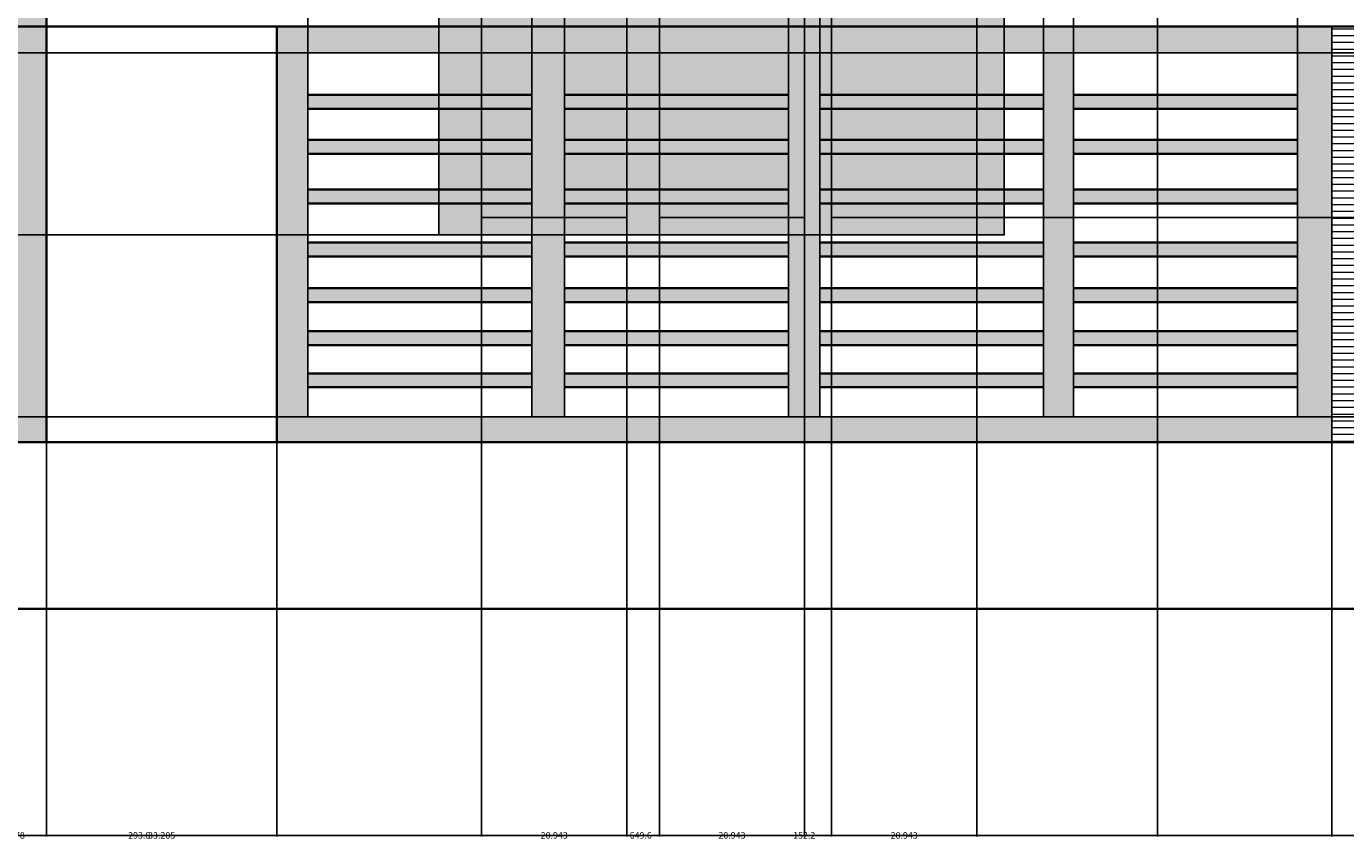
# Model space of a CAD drawing. Units: inches. Extents: x -5 to 714, y 84 to 644.
# Tile 5 of 20: x 266 to 457, y 84 to 201. Entities that reach past the tile are written whole.
import ezdxf

# ---------------------------------------------------------------- set-up
doc = ezdxf.new("R2010")
doc.units = ezdxf.units.IN
doc.header["$MEASUREMENT"] = 0
for name, color, linetype, lineweight in [('A-ANNO-DIMS', 2, 'Continuous', 18), ('A-ELEV', 7, 'Continuous', 35), ('A-ELEV-PATT', 8, 'Continuous', 13), ('A-GLAZ', 3, 'Continuous', 25)]:
    doc.layers.add(name, color=color, linetype=linetype, lineweight=lineweight)
doc.styles.get("Standard").update_dxf_attribs({"font": 'arial.ttf'})
doc.dimstyles.get("Standard").update_dxf_attribs({"dimtxt": 0.9375, "dimasz": 0.18, "dimexe": 0.18, "dimexo": 0.0625, "dimgap": 0.09, "dimtad": 0, "dimtih": 1, "dimtoh": 1, "dimdec": 4, "dimzin": 0, "dimdsep": 46, "dimlunit": 4, "dimtxsty": 'Standard', "dimcen": 0.09, "dimadec": 0, "dimazin": 0, "dimtfac": 1, "dimtdec": 4, "dimtofl": 0, "dimtmove": 0, "dimatfit": 3, "dimfxl": 1, "dimtolj": 1, "dimtzin": 0, "dimarcsym": 0})

# ---------------------------------------------------------------- blocks, each defined once
blk = doc.blocks.new('*D1')
at = {"layer": 'A-ANNO-DIMS', "color": 0, "lineweight": -2, "transparency": 16777216}
for p, q in [((30.14, 117.13), (30.14, 84.31)), ((679.78, 117.13), (679.78, 84.31)), ((30.32, 84.49), (353.29, 84.49)), ((679.6, 84.49), (356.64, 84.49))]:
    blk.add_line(p, q, dxfattribs=at)
at = {"layer": 'A-ANNO-DIMS', "color": 0, "transparency": 16777216}
for points in [[(30.32, 84.52), (30.32, 84.46), (30.14, 84.49)], [(679.6, 84.52), (679.6, 84.46), (679.78, 84.49)]]:
    blk.add_solid(points, dxfattribs=at)
at = {"layer": 'Defpoints', "color": 0, "transparency": 16777216}
for p in [(30.14, 117.19), (679.78, 117.19), (679.78, 84.49)]:
    blk.add_point(p, dxfattribs=at)
at = {"layer": 'A-ANNO-DIMS', "color": 0, "transparency": 16777216, "insert": (354.96, 84.49), "char_height": 0.938, "attachment_point": 5}
blk.add_mtext('\\A1;649.6', dxfattribs=at)
blk = doc.blocks.new('*D29')
at = {"layer": 'A-ANNO-DIMS', "color": 0, "lineweight": -2, "transparency": 16777216}
for p, q in [((135.73, 471.11), (135.73, 84.31)), ((429.51, 471.11), (429.51, 84.31)), ((135.91, 84.49), (280.94, 84.49)), ((429.33, 84.49), (284.3, 84.49))]:
    blk.add_line(p, q, dxfattribs=at)
at = {"layer": 'A-ANNO-DIMS', "color": 0, "transparency": 16777216}
for points in [[(135.91, 84.52), (135.91, 84.46), (135.73, 84.49)], [(429.33, 84.52), (429.33, 84.46), (429.51, 84.49)]]:
    blk.add_solid(points, dxfattribs=at)
at = {"layer": 'Defpoints', "color": 0, "transparency": 16777216}
for p in [(135.73, 471.17), (429.51, 471.17), (429.51, 84.49)]:
    blk.add_point(p, dxfattribs=at)
at = {"layer": 'A-ANNO-DIMS', "color": 0, "transparency": 16777216, "insert": (282.62, 84.49), "char_height": 0.938, "attachment_point": 5}
blk.add_mtext('\\A1;293.8', dxfattribs=at)
blk = doc.blocks.new('*D53')
at = {"layer": 'A-ANNO-DIMS', "color": 0, "lineweight": -2, "transparency": 16777216}
for p, q in [((259.07, 315.03), (259.07, 84.31)), ((269.24, 306.57), (269.24, 84.31)), ((259.25, 84.49), (262.16, 84.49)), ((269.06, 84.49), (266.15, 84.49))]:
    blk.add_line(p, q, dxfattribs=at)
at = {"layer": 'A-ANNO-DIMS', "color": 0, "transparency": 16777216}
for points in [[(259.25, 84.52), (259.25, 84.46), (259.07, 84.49)], [(269.06, 84.52), (269.06, 84.46), (269.24, 84.49)]]:
    blk.add_solid(points, dxfattribs=at)
at = {"layer": 'Defpoints', "color": 0, "transparency": 16777216}
for p in [(259.07, 315.1), (269.24, 306.63), (269.24, 84.49)]:
    blk.add_point(p, dxfattribs=at)
at = {"layer": 'A-ANNO-DIMS', "color": 0, "transparency": 16777216, "insert": (264.16, 84.49), "char_height": 0.938, "attachment_point": 5}
blk.add_mtext('\\A1;10.178', dxfattribs=at)
blk = doc.blocks.new('*D65')
at = {"layer": 'A-ANNO-DIMS', "color": 0, "lineweight": -2, "transparency": 16777216}
for p, q in [((325.77, 266), (-2.74, 266)), ((-2.56, 265.82), (-2.56, 219.13)), ((-2.56, 171.3), (-2.56, 217.99)), ((325.77, 171.12), (-2.74, 171.12))]:
    blk.add_line(p, q, dxfattribs=at)
at = {"layer": 'A-ANNO-DIMS', "color": 0, "transparency": 16777216}
for points in [[(-2.59, 265.82), (-2.53, 265.82), (-2.56, 266)], [(-2.59, 171.3), (-2.53, 171.3), (-2.56, 171.12)]]:
    blk.add_solid(points, dxfattribs=at)
at = {"layer": 'Defpoints', "color": 0, "transparency": 16777216}
for p in [(-2.56, 266), (325.83, 266), (325.83, 171.12)]:
    blk.add_point(p, dxfattribs=at)
at = {"layer": 'A-ANNO-DIMS', "color": 0, "transparency": 16777216, "insert": (-2.56, 218.56), "char_height": 0.938, "attachment_point": 5}
blk.add_mtext('\\A1;94.88', dxfattribs=at)
blk = doc.blocks.new('*D66')
at = {"layer": 'A-ANNO-DIMS', "color": 0, "lineweight": -2, "transparency": 16777216}
for p, q in [((332.01, 258.22), (332.01, 84.31)), ((352.95, 258.22), (352.95, 84.31)), ((332.19, 84.49), (340.43, 84.49)), ((352.77, 84.49), (344.52, 84.49))]:
    blk.add_line(p, q, dxfattribs=at)
at = {"layer": 'A-ANNO-DIMS', "color": 0, "transparency": 16777216}
for points in [[(332.19, 84.52), (332.19, 84.46), (332.01, 84.49)], [(352.77, 84.52), (352.77, 84.46), (352.95, 84.49)]]:
    blk.add_solid(points, dxfattribs=at)
at = {"layer": 'Defpoints', "color": 0, "transparency": 16777216}
for p in [(332.01, 258.29), (352.95, 258.29), (352.95, 84.49)]:
    blk.add_point(p, dxfattribs=at)
at = {"layer": 'A-ANNO-DIMS', "color": 0, "transparency": 16777216, "insert": (342.48, 84.49), "char_height": 0.938, "attachment_point": 5}
blk.add_mtext('\\A1;20.943', dxfattribs=at)
blk = doc.blocks.new('*D67')
at = {"layer": 'A-ANNO-DIMS', "color": 0, "lineweight": -2, "transparency": 16777216}
for p, q in [((357.65, 258.22), (357.65, 84.31)), ((378.6, 258.22), (378.6, 84.31)), ((357.83, 84.49), (366.08, 84.49)), ((378.42, 84.49), (370.17, 84.49))]:
    blk.add_line(p, q, dxfattribs=at)
at = {"layer": 'A-ANNO-DIMS', "color": 0, "transparency": 16777216}
for points in [[(357.83, 84.52), (357.83, 84.46), (357.65, 84.49)], [(378.42, 84.52), (378.42, 84.46), (378.6, 84.49)]]:
    blk.add_solid(points, dxfattribs=at)
at = {"layer": 'Defpoints', "color": 0, "transparency": 16777216}
for p in [(357.65, 258.29), (378.6, 258.29), (378.6, 84.49)]:
    blk.add_point(p, dxfattribs=at)
at = {"layer": 'A-ANNO-DIMS', "color": 0, "transparency": 16777216, "insert": (368.12, 84.49), "char_height": 0.938, "attachment_point": 5}
blk.add_mtext('\\A1;20.943', dxfattribs=at)
blk = doc.blocks.new('*D68')
at = {"layer": 'A-ANNO-DIMS', "color": 0, "lineweight": -2, "transparency": 16777216}
for p, q in [((382.5, 258.22), (382.5, 84.31)), ((403.44, 258.22), (403.44, 84.31)), ((382.68, 84.49), (390.92, 84.49)), ((403.26, 84.49), (395.01, 84.49))]:
    blk.add_line(p, q, dxfattribs=at)
at = {"layer": 'A-ANNO-DIMS', "color": 0, "transparency": 16777216}
for points in [[(382.68, 84.52), (382.68, 84.46), (382.5, 84.49)], [(403.26, 84.52), (403.26, 84.46), (403.44, 84.49)]]:
    blk.add_solid(points, dxfattribs=at)
at = {"layer": 'Defpoints', "color": 0, "transparency": 16777216}
for p in [(382.5, 258.29), (403.44, 258.29), (403.44, 84.49)]:
    blk.add_point(p, dxfattribs=at)
at = {"layer": 'A-ANNO-DIMS', "color": 0, "transparency": 16777216, "insert": (392.97, 84.49), "char_height": 0.938, "attachment_point": 5}
blk.add_mtext('\\A1;20.943', dxfattribs=at)
blk = doc.blocks.new('*D69')
at = {"layer": 'A-ANNO-DIMS', "color": 0, "lineweight": -2, "transparency": 16777216}
for p, q in [((403.5, 258.29), (712.66, 258.29)), ((712.48, 258.11), (712.48, 216.52)), ((712.48, 173.8), (712.48, 215.38)), ((403.5, 173.62), (712.66, 173.62))]:
    blk.add_line(p, q, dxfattribs=at)
at = {"layer": 'A-ANNO-DIMS', "color": 0, "transparency": 16777216}
for points in [[(712.45, 258.11), (712.51, 258.11), (712.48, 258.29)], [(712.45, 173.8), (712.51, 173.8), (712.48, 173.62)]]:
    blk.add_solid(points, dxfattribs=at)
at = {"layer": 'Defpoints', "color": 0, "transparency": 16777216}
for p in [(403.44, 258.29), (712.48, 258.29), (403.44, 173.62)]:
    blk.add_point(p, dxfattribs=at)
at = {"layer": 'A-ANNO-DIMS', "color": 0, "transparency": 16777216, "insert": (712.48, 215.95), "char_height": 0.938, "attachment_point": 5}
blk.add_mtext('\\A1;84.67', dxfattribs=at)
blk = doc.blocks.new('*D74')
at = {"layer": 'A-ANNO-DIMS', "color": 0, "lineweight": -2, "transparency": 16777216}
for p, q in [((179.93, 141.13), (179.93, 84.31)), ((269.24, 141.13), (269.24, 84.31)), ((180.11, 84.49), (223.01, 84.49)), ((269.06, 84.49), (226.17, 84.49))]:
    blk.add_line(p, q, dxfattribs=at)
at = {"layer": 'A-ANNO-DIMS', "color": 0, "transparency": 16777216}
for points in [[(180.11, 84.52), (180.11, 84.46), (179.93, 84.49)], [(269.06, 84.52), (269.06, 84.46), (269.24, 84.49)]]:
    blk.add_solid(points, dxfattribs=at)
at = {"layer": 'Defpoints', "color": 0, "transparency": 16777216}
for p in [(179.93, 141.19), (269.24, 141.19), (269.24, 84.49)]:
    blk.add_point(p, dxfattribs=at)
at = {"layer": 'A-ANNO-DIMS', "color": 0, "transparency": 16777216, "insert": (224.59, 84.49), "char_height": 0.938, "attachment_point": 5}
blk.add_mtext('\\A1;89.31', dxfattribs=at)
blk = doc.blocks.new('*D75')
at = {"layer": 'A-ANNO-DIMS', "color": 0, "lineweight": -2, "transparency": 16777216}
for p, q in [((269.24, 141.13), (269.24, 84.31)), ((302.45, 141.13), (302.45, 84.31)), ((269.42, 84.49), (283.81, 84.49)), ((302.27, 84.49), (287.89, 84.49))]:
    blk.add_line(p, q, dxfattribs=at)
at = {"layer": 'A-ANNO-DIMS', "color": 0, "transparency": 16777216}
for points in [[(269.42, 84.52), (269.42, 84.46), (269.24, 84.49)], [(302.27, 84.52), (302.27, 84.46), (302.45, 84.49)]]:
    blk.add_solid(points, dxfattribs=at)
at = {"layer": 'Defpoints', "color": 0, "transparency": 16777216}
for p in [(269.24, 141.19), (302.45, 141.19), (302.45, 84.49)]:
    blk.add_point(p, dxfattribs=at)
at = {"layer": 'A-ANNO-DIMS', "color": 0, "transparency": 16777216, "insert": (285.85, 84.49), "char_height": 0.938, "attachment_point": 5}
blk.add_mtext('\\A1;33.205', dxfattribs=at)
blk = doc.blocks.new('*D76')
at = {"layer": 'A-ANNO-DIMS', "color": 0, "lineweight": -2, "transparency": 16777216}
for p, q in [((302.45, 141.13), (302.45, 84.31)), ((454.64, 141.13), (454.64, 84.31)), ((302.63, 84.49), (376.92, 84.49)), ((454.46, 84.49), (380.17, 84.49))]:
    blk.add_line(p, q, dxfattribs=at)
at = {"layer": 'A-ANNO-DIMS', "color": 0, "transparency": 16777216}
for points in [[(302.63, 84.52), (302.63, 84.46), (302.45, 84.49)], [(454.46, 84.52), (454.46, 84.46), (454.64, 84.49)]]:
    blk.add_solid(points, dxfattribs=at)
at = {"layer": 'Defpoints', "color": 0, "transparency": 16777216}
for p in [(302.45, 141.19), (454.64, 141.19), (454.64, 84.49)]:
    blk.add_point(p, dxfattribs=at)
at = {"layer": 'A-ANNO-DIMS', "color": 0, "transparency": 16777216, "insert": (378.55, 84.49), "char_height": 0.938, "attachment_point": 5}
blk.add_mtext('\\A1;152.2', dxfattribs=at)
blk = doc.blocks.new('*D77')
at = {"layer": 'A-ANNO-DIMS', "color": 0, "lineweight": -2, "transparency": 16777216}
for p, q in [((454.64, 141.13), (454.64, 84.31)), ((493.78, 141.13), (493.78, 84.31)), ((454.82, 84.49), (472.54, 84.49)), ((493.6, 84.49), (475.88, 84.49))]:
    blk.add_line(p, q, dxfattribs=at)
at = {"layer": 'A-ANNO-DIMS', "color": 0, "transparency": 16777216}
for points in [[(454.82, 84.52), (454.82, 84.46), (454.64, 84.49)], [(493.6, 84.52), (493.6, 84.46), (493.78, 84.49)]]:
    blk.add_solid(points, dxfattribs=at)
at = {"layer": 'Defpoints', "color": 0, "transparency": 16777216}
for p in [(454.64, 141.19), (493.78, 141.19), (493.78, 84.49)]:
    blk.add_point(p, dxfattribs=at)
at = {"layer": 'A-ANNO-DIMS', "color": 0, "transparency": 16777216, "insert": (474.21, 84.49), "char_height": 0.938, "attachment_point": 5}
blk.add_mtext('\\A1;39.13', dxfattribs=at)
blk = doc.blocks.new('*D83')
at = {"layer": 'A-ANNO-DIMS', "color": 0, "lineweight": -2, "transparency": 16777216}
for p, q in [((306.96, 144.93), (306.96, 643.61)), ((307.14, 643.43), (321.53, 643.43)), ((339.09, 643.43), (324.69, 643.43)), ((339.27, 144.93), (339.27, 643.61))]:
    blk.add_line(p, q, dxfattribs=at)
at = {"layer": 'A-ANNO-DIMS', "color": 0, "transparency": 16777216}
for points in [[(307.14, 643.46), (307.14, 643.4), (306.96, 643.43)], [(339.09, 643.46), (339.09, 643.4), (339.27, 643.43)]]:
    blk.add_solid(points, dxfattribs=at)
at = {"layer": 'Defpoints', "color": 0, "transparency": 16777216}
for p in [(339.27, 643.43), (306.96, 144.86), (339.27, 144.86)]:
    blk.add_point(p, dxfattribs=at)
at = {"layer": 'A-ANNO-DIMS', "color": 0, "transparency": 16777216, "insert": (323.11, 643.43), "char_height": 0.938, "attachment_point": 5}
blk.add_mtext('\\A1;32.31', dxfattribs=at)
blk = doc.blocks.new('*D84')
at = {"layer": 'A-ANNO-DIMS', "color": 0, "lineweight": -2, "transparency": 16777216}
for p, q in [((343.97, 144.93), (343.97, 643.61)), ((344.15, 643.43), (358.54, 643.43)), ((376.1, 643.43), (361.71, 643.43)), ((376.28, 144.93), (376.28, 643.61))]:
    blk.add_line(p, q, dxfattribs=at)
at = {"layer": 'A-ANNO-DIMS', "color": 0, "transparency": 16777216}
for points in [[(344.15, 643.46), (344.15, 643.4), (343.97, 643.43)], [(376.1, 643.46), (376.1, 643.4), (376.28, 643.43)]]:
    blk.add_solid(points, dxfattribs=at)
at = {"layer": 'Defpoints', "color": 0, "transparency": 16777216}
for p in [(376.28, 643.43), (343.97, 144.86), (376.28, 144.86)]:
    blk.add_point(p, dxfattribs=at)
at = {"layer": 'A-ANNO-DIMS', "color": 0, "transparency": 16777216, "insert": (360.13, 643.43), "char_height": 0.938, "attachment_point": 5}
blk.add_mtext('\\A1;32.31', dxfattribs=at)
blk = doc.blocks.new('*D85')
at = {"layer": 'A-ANNO-DIMS', "color": 0, "lineweight": -2, "transparency": 16777216}
for p, q in [((380.78, 144.93), (380.78, 643.61)), ((380.96, 643.43), (395.35, 643.43)), ((412.91, 643.43), (398.51, 643.43)), ((413.09, 144.93), (413.09, 643.61))]:
    blk.add_line(p, q, dxfattribs=at)
at = {"layer": 'A-ANNO-DIMS', "color": 0, "transparency": 16777216}
for points in [[(380.96, 643.46), (380.96, 643.4), (380.78, 643.43)], [(412.91, 643.46), (412.91, 643.4), (413.09, 643.43)]]:
    blk.add_solid(points, dxfattribs=at)
at = {"layer": 'Defpoints', "color": 0, "transparency": 16777216}
for p in [(413.09, 643.43), (380.78, 144.86), (413.09, 144.86)]:
    blk.add_point(p, dxfattribs=at)
at = {"layer": 'A-ANNO-DIMS', "color": 0, "transparency": 16777216, "insert": (396.93, 643.43), "char_height": 0.938, "attachment_point": 5}
blk.add_mtext('\\A1;32.31', dxfattribs=at)
blk = doc.blocks.new('*D86')
at = {"layer": 'A-ANNO-DIMS', "color": 0, "lineweight": -2, "transparency": 16777216}
for p, q in [((417.38, 144.93), (417.38, 643.61)), ((417.56, 643.43), (431.96, 643.43)), ((449.51, 643.43), (435.12, 643.43)), ((449.69, 144.93), (449.69, 643.61))]:
    blk.add_line(p, q, dxfattribs=at)
at = {"layer": 'A-ANNO-DIMS', "color": 0, "transparency": 16777216}
for points in [[(417.56, 643.46), (417.56, 643.4), (417.38, 643.43)], [(449.51, 643.46), (449.51, 643.4), (449.69, 643.43)]]:
    blk.add_solid(points, dxfattribs=at)
at = {"layer": 'Defpoints', "color": 0, "transparency": 16777216}
for p in [(449.69, 643.43), (417.38, 144.86), (449.69, 144.86)]:
    blk.add_point(p, dxfattribs=at)
at = {"layer": 'A-ANNO-DIMS', "color": 0, "transparency": 16777216, "insert": (433.54, 643.43), "char_height": 0.938, "attachment_point": 5}
blk.add_mtext('\\A1;32.31', dxfattribs=at)
blk = doc.blocks.new('*D87')
at = {"layer": 'A-ANNO-DIMS', "color": 0, "lineweight": -2, "transparency": 16777216}
for p, q in [((306.9, 197.38), (-2.74, 197.38)), ((-2.56, 197.2), (-2.56, 171.69)), ((-2.56, 145.04), (-2.56, 170.55)), ((306.9, 144.86), (-2.74, 144.86))]:
    blk.add_line(p, q, dxfattribs=at)
at = {"layer": 'A-ANNO-DIMS', "color": 0, "transparency": 16777216}
for points in [[(-2.59, 197.2), (-2.53, 197.2), (-2.56, 197.38)], [(-2.59, 145.04), (-2.53, 145.04), (-2.56, 144.86)]]:
    blk.add_solid(points, dxfattribs=at)
at = {"layer": 'Defpoints', "color": 0, "transparency": 16777216}
for p in [(-2.56, 197.38), (306.96, 197.38), (306.96, 144.86)]:
    blk.add_point(p, dxfattribs=at)
at = {"layer": 'A-ANNO-DIMS', "color": 0, "transparency": 16777216, "insert": (-2.56, 171.12), "char_height": 0.938, "attachment_point": 5}
blk.add_mtext('\\A1;52.51', dxfattribs=at)
blk = doc.blocks.new('*D89')
at = {"layer": 'A-ANNO-DIMS', "color": 0, "lineweight": -2, "transparency": 16777216}
for p, q in [((541.31, 197.38), (-2.74, 197.38)), ((-2.56, 197.2), (-2.56, 171.69)), ((-2.56, 145.04), (-2.56, 170.55)), ((541.31, 144.86), (-2.74, 144.86))]:
    blk.add_line(p, q, dxfattribs=at)
at = {"layer": 'A-ANNO-DIMS', "color": 0, "transparency": 16777216}
for points in [[(-2.59, 197.2), (-2.53, 197.2), (-2.56, 197.38)], [(-2.59, 145.04), (-2.53, 145.04), (-2.56, 144.86)]]:
    blk.add_solid(points, dxfattribs=at)
at = {"layer": 'Defpoints', "color": 0, "transparency": 16777216}
for p in [(-2.56, 197.38), (541.38, 197.38), (541.38, 144.86)]:
    blk.add_point(p, dxfattribs=at)
at = {"layer": 'A-ANNO-DIMS', "color": 0, "transparency": 16777216, "insert": (-2.56, 171.12), "char_height": 0.938, "attachment_point": 5}
blk.add_mtext('\\A1;52.51', dxfattribs=at)

msp = doc.modelspace()

# ---------------------------------------------------------------- hatches: boundary and pattern name
at = {"layer": 'A-ELEV-PATT', "transparency": 33554687}
h = msp.add_hatch(color=256, dxfattribs=at)
h.dxf.hatch_style = 1
h.paths.add_polyline_path([(188.3677, 525.1928), (67.9893, 525.1928), (67.9893, 489.1928), (67.9893, 345.1928), (126.7303, 345.1928), (126.7303, 480.1709), (229.3575, 480.1709), (229.3575, 525.1928), (212.6043, 525.1928), (212.6043, 482.7164), (211.0019, 482.7164), (211.0019, 525.1928), (207.6919, 525.1928), (199.9852, 525.1928), (199.9852, 482.7164), (198.3828, 482.7164), (198.3828, 525.1928), (189.9701, 525.1928), (189.9701, 482.7164), (188.3677, 482.7164)])
h.paths.add_polyline_path([(121.3589, 336.2066), (75.5048, 336.2066), (75.5048, 319.345), (121.3589, 319.345)])
h.paths.add_polyline_path([(121.3589, 319.345), (75.5048, 319.345), (75.5048, 302.3045), (121.3589, 302.3045)])
h.paths.add_polyline_path([(121.3589, 302.3045), (75.5048, 302.3045), (75.5048, 282.8561), (121.3589, 282.8561)])
h.paths.add_polyline_path([(121.3589, 282.8561), (75.5048, 282.8561), (75.5048, 261.5556), (121.3589, 261.5556)])
h.paths.add_polyline_path([(121.3589, 261.5556), (75.5048, 261.5556), (75.5048, 243.7009), (121.3589, 243.7009)])
h.paths.add_polyline_path([(121.3589, 243.7009), (75.5048, 243.7009), (75.5048, 223.5117), (121.3589, 223.5117)])
h.paths.add_polyline_path([(121.3589, 223.5117), (75.5048, 223.5117), (75.5048, 212.5836), (121.3589, 212.5836)])
h.paths.add_polyline_path([(121.3589, 212.5836), (75.5048, 212.5836), (75.5048, 201.1928), (121.3589, 201.1928)])
h.paths.add_polyline_path([(179.9335, 201.1928), (30.1395, 201.1928), (30.1395, 198.7054), (179.9335, 198.7054)])
h.paths.add_polyline_path([(187.6349, 201.1928), (179.9335, 201.1928), (179.9335, 198.7054), (179.9335, 141.1928), (269.2446, 141.1928), (269.2446, 201.1928), (263.4349, 201.1928), (263.4349, 152.1176), (187.6349, 152.1176)])
h.paths.add_polyline_path([(269.2446, 277.0513), (269.2446, 287.501), (269.2446, 306.6286), (578.0915, 306.6286), (578.0915, 201.1928), (593.428, 201.1928), (593.428, 315.0968), (584.4202, 315.0968), (259.0665, 315.0968), (259.0665, 201.1928), (263.4349, 201.1928), (269.2446, 201.1928)])
h = msp.add_hatch(color=256, dxfattribs=at)
h.dxf.hatch_style = 1
h.paths.add_polyline_path([(584.2229, 343.1928), (259.0665, 343.1928), (259.0665, 315.0968), (584.2229, 315.0968)])
h.paths.add_polyline_path([(352.9482, 258.2864), (332.0052, 258.2864), (332.0052, 201.1928), (352.9482, 201.1928)])
h.paths.add_polyline_path([(378.5957, 258.2864), (357.6527, 258.2864), (357.6527, 201.1928), (378.5957, 201.1928)])
h.paths.add_polyline_path([(403.4391, 258.2864), (382.4961, 258.2864), (382.4961, 201.1928), (403.4391, 201.1928)])
h.paths.add_polyline_path([(339.2672, 197.3754), (332.0052, 197.3754), (332.0052, 191.3028), (339.2672, 191.3028)])
h.paths.add_polyline_path([(352.9482, 197.3754), (343.9704, 197.3754), (343.9704, 191.3028), (352.9482, 191.3028)])
h.paths.add_polyline_path([(352.9482, 189.3028), (343.9704, 189.3028), (343.9704, 184.8307), (352.9482, 184.8307)])
h.paths.add_polyline_path([(339.2672, 189.3028), (332.0052, 189.3028), (332.0052, 184.8307), (339.2672, 184.8307)])
h.paths.add_polyline_path([(339.2672, 182.8307), (332.0052, 182.8307), (332.0052, 177.6504), (339.2672, 177.6504)])
h.paths.add_polyline_path([(352.9482, 182.8307), (343.9704, 182.8307), (343.9704, 177.6504), (352.9482, 177.6504)])
h.paths.add_polyline_path([(352.9482, 175.6504), (343.9704, 175.6504), (343.9704, 173.6169), (352.9482, 173.6169)])
h.paths.add_polyline_path([(339.2672, 175.6504), (332.0052, 175.6504), (332.0052, 173.6169), (339.2672, 173.6169)])
h.paths.add_polyline_path([(376.2796, 175.6504), (357.6527, 175.6504), (357.6527, 173.6169), (376.2796, 173.6169)])
h.paths.add_polyline_path([(376.2796, 182.8307), (357.6527, 182.8307), (357.6527, 177.6504), (376.2796, 177.6504)])
h.paths.add_polyline_path([(376.2796, 189.3028), (357.6527, 189.3028), (357.6527, 184.8307), (376.2796, 184.8307)])
h.paths.add_polyline_path([(376.2796, 197.3754), (357.6527, 197.3754), (357.6527, 191.3028), (376.2796, 191.3028)])
h.paths.add_polyline_path([(403.4391, 197.3754), (382.4961, 197.3754), (382.4961, 191.3028), (403.4391, 191.3028)])
h.paths.add_polyline_path([(403.4391, 189.3028), (382.4961, 189.3028), (382.4961, 184.8307), (403.4391, 184.8307)])
h.paths.add_polyline_path([(403.4391, 182.8307), (382.4961, 182.8307), (382.4961, 177.6504), (403.4391, 177.6504)])
h.paths.add_polyline_path([(403.4391, 175.6504), (382.4961, 175.6504), (382.4961, 173.6169), (403.4391, 173.6169)])
h = msp.add_hatch(color=256, dxfattribs=at)
h.dxf.hatch_style = 1
h.paths.add_polyline_path([(407.3813, 266.0021), (325.8305, 266.0021), (325.8305, 201.1928), (332.0052, 201.1928), (332.0052, 258.2864), (352.9482, 258.2864), (352.9482, 201.1928), (357.6527, 201.1928), (357.6527, 258.2864), (378.5957, 258.2864), (378.5957, 201.1928), (382.4961, 201.1928), (382.4961, 258.2864), (403.4391, 258.2864), (403.4391, 201.1928), (407.3813, 201.1928)])
h = msp.add_hatch(color=256, dxfattribs=at)
h.dxf.hatch_style = 1
h.paths.add_polyline_path([(499.6809, 257.3379), (537.1779, 257.3379), (537.1779, 201.1928), (543.7164, 201.1928), (543.7164, 266.0021), (493.7771, 266.0021), (493.7771, 201.1928), (499.6809, 201.1928)])
h.paths.add_polyline_path([(407.3813, 197.3754), (403.4391, 197.3754), (403.4391, 191.3028), (407.3813, 191.3028)])
h.paths.add_polyline_path([(407.3813, 189.3028), (403.4391, 189.3028), (403.4391, 184.8307), (407.3813, 184.8307)])
h.paths.add_polyline_path([(407.3813, 182.8307), (403.4391, 182.8307), (403.4391, 177.6504), (407.3813, 177.6504)])
h.paths.add_polyline_path([(407.3813, 175.6504), (403.4391, 175.6504), (403.4391, 173.6169), (382.4961, 173.6169), (382.4961, 175.6504), (380.7784, 175.6504), (380.7784, 171.1197), (407.3813, 171.1197)])
h.paths.add_polyline_path([(382.4961, 182.8307), (380.7784, 182.8307), (380.7784, 177.6504), (382.4961, 177.6504)])
h.paths.add_polyline_path([(382.4961, 189.3028), (380.7784, 189.3028), (380.7784, 184.8307), (382.4961, 184.8307)])
h.paths.add_polyline_path([(382.4961, 197.3754), (380.7784, 197.3754), (380.7784, 191.3028), (382.4961, 191.3028)])
h.paths.add_polyline_path([(357.6527, 197.3754), (352.9482, 197.3754), (352.9482, 191.3028), (357.6527, 191.3028)])
h.paths.add_polyline_path([(357.6527, 189.3028), (352.9482, 189.3028), (352.9482, 184.8307), (357.6527, 184.8307)])
h.paths.add_polyline_path([(357.6527, 182.8307), (352.9482, 182.8307), (352.9482, 177.6504), (357.6527, 177.6504)])
h.paths.add_polyline_path([(376.2796, 173.6169), (357.6527, 173.6169), (357.6527, 175.6504), (352.9482, 175.6504), (352.9482, 173.6169), (343.9704, 173.6169), (343.9704, 171.1197), (376.2796, 171.1197)])
h.paths.add_polyline_path([(339.2672, 173.6169), (332.0052, 173.6169), (332.0052, 175.6504), (325.8305, 175.6504), (325.8305, 171.1197), (339.2672, 171.1197)])
h.paths.add_polyline_path([(332.0052, 182.8307), (325.8305, 182.8307), (325.8305, 177.6504), (332.0052, 177.6504)])
h.paths.add_polyline_path([(332.0052, 189.3028), (325.8305, 189.3028), (325.8305, 184.8307), (332.0052, 184.8307)])
h.paths.add_polyline_path([(332.0052, 197.3754), (325.8305, 197.3754), (325.8305, 191.3028), (332.0052, 191.3028)])
h = msp.add_hatch(color=256, dxfattribs=at)
h.dxf.hatch_style = 1
h.paths.add_polyline_path([(449.6911, 151.1385), (417.3818, 151.1385), (417.3818, 149.1385), (449.6911, 149.1385)])
h.paths.add_polyline_path([(449.6911, 157.2254), (417.3818, 157.2254), (417.3818, 155.2254), (449.6911, 155.2254)])
h.paths.add_polyline_path([(449.6911, 163.4201), (417.3818, 163.4201), (417.3818, 161.4201), (449.6911, 161.4201)])
h.paths.add_polyline_path([(449.6911, 170.0006), (417.3818, 170.0006), (417.3818, 168.0006), (449.6911, 168.0006)])
h.paths.add_polyline_path([(449.6911, 177.6504), (417.3818, 177.6504), (417.3818, 175.6504), (449.6911, 175.6504)])
h.paths.add_polyline_path([(449.6911, 184.8307), (417.3818, 184.8307), (417.3818, 182.8307), (449.6911, 182.8307)])
h.paths.add_polyline_path([(449.6911, 191.3028), (417.3818, 191.3028), (417.3818, 189.3028), (449.6911, 189.3028)])
h.paths.add_polyline_path([(407.3813, 191.3028), (403.4391, 191.3028), (403.4391, 189.3028), (407.3813, 189.3028)])
h.paths.add_polyline_path([(413.0876, 191.3028), (407.3813, 191.3028), (407.3813, 189.3028), (413.0876, 189.3028)])
h.paths.add_polyline_path([(403.4391, 191.3028), (382.4961, 191.3028), (382.4961, 189.3028), (403.4391, 189.3028)])
h.paths.add_polyline_path([(403.4391, 184.8307), (382.4961, 184.8307), (382.4961, 182.8307), (403.4391, 182.8307)])
h.paths.add_polyline_path([(403.4391, 177.6504), (382.4961, 177.6504), (382.4961, 175.6504), (403.4391, 175.6504)])
h.paths.add_polyline_path([(382.4961, 177.6504), (380.7784, 177.6504), (380.7784, 175.6504), (382.4961, 175.6504)], flags=17)
h.paths.add_polyline_path([(343.9704, 173.6169), (339.2672, 173.6169), (339.2672, 171.1197), (343.9704, 171.1197)])
h.paths.add_polyline_path([(343.9704, 197.3754), (352.9482, 197.3754), (352.9482, 258.2864), (332.0052, 258.2864), (332.0052, 197.3754), (339.2672, 197.3754), (339.2672, 173.6169), (343.9704, 173.6169)])
h.paths.add_polyline_path([(339.2672, 191.3028), (332.0052, 191.3028), (332.0052, 189.3028), (339.2672, 189.3028)], flags=17)
h.paths.add_polyline_path([(332.0052, 191.3028), (325.8305, 191.3028), (325.8305, 189.3028), (332.0052, 189.3028)])
h.paths.add_polyline_path([(332.0052, 201.1928), (325.8305, 201.1928), (325.8305, 197.3754), (332.0052, 197.3754)])
h.paths.add_polyline_path([(357.6527, 201.1928), (352.9482, 201.1928), (352.9482, 197.3754), (357.6527, 197.3754)])
h.paths.add_polyline_path([(378.5957, 201.1928), (357.6527, 201.1928), (357.6527, 197.3754), (376.2796, 197.3754), (376.2796, 173.6169), (378.5957, 173.6169)])
h.paths.add_polyline_path([(382.4961, 201.1928), (378.5957, 201.1928), (378.5957, 173.6169), (376.2796, 173.6169), (376.2796, 171.1197), (380.7784, 171.1197), (380.7784, 197.3754), (382.4961, 197.3754)])
h.paths.add_polyline_path([(403.4391, 201.1928), (382.4961, 201.1928), (382.4961, 197.3754), (403.4391, 197.3754)])
h.paths.add_polyline_path([(407.3813, 201.1928), (403.4391, 201.1928), (403.4391, 197.3754), (407.3813, 197.3754)])
h.paths.add_polyline_path([(352.9482, 191.3028), (343.9704, 191.3028), (343.9704, 189.3028), (352.9482, 189.3028)], flags=17)
h.paths.add_polyline_path([(376.2796, 191.3028), (357.6527, 191.3028), (357.6527, 189.3028), (376.2796, 189.3028)], flags=17)
h.paths.add_polyline_path([(332.0052, 184.8307), (325.8305, 184.8307), (325.8305, 182.8307), (332.0052, 182.8307)])
h.paths.add_polyline_path([(339.2672, 184.8307), (332.0052, 184.8307), (332.0052, 182.8307), (339.2672, 182.8307)], flags=17)
h.paths.add_polyline_path([(352.9482, 184.8307), (343.9704, 184.8307), (343.9704, 182.8307), (352.9482, 182.8307)], flags=17)
h.paths.add_polyline_path([(357.6527, 191.3028), (352.9482, 191.3028), (352.9482, 189.3028), (357.6527, 189.3028)])
h.paths.add_polyline_path([(357.6527, 184.8307), (352.9482, 184.8307), (352.9482, 182.8307), (357.6527, 182.8307)])
h.paths.add_polyline_path([(376.2796, 184.8307), (357.6527, 184.8307), (357.6527, 182.8307), (376.2796, 182.8307)], flags=17)
h.paths.add_polyline_path([(357.6527, 177.6504), (352.9482, 177.6504), (352.9482, 175.6504), (357.6527, 175.6504)])
h.paths.add_polyline_path([(376.2796, 177.6504), (357.6527, 177.6504), (357.6527, 175.6504), (376.2796, 175.6504)], flags=17)
h.paths.add_polyline_path([(352.9482, 177.6504), (343.9704, 177.6504), (343.9704, 175.6504), (352.9482, 175.6504)], flags=17)
h.paths.add_polyline_path([(339.2672, 177.6504), (332.0052, 177.6504), (332.0052, 175.6504), (339.2672, 175.6504)], flags=17)
h.paths.add_polyline_path([(332.0052, 177.6504), (325.8305, 177.6504), (325.8305, 175.6504), (332.0052, 175.6504)])
h.paths.add_polyline_path([(382.4961, 191.3028), (380.7784, 191.3028), (380.7784, 189.3028), (382.4961, 189.3028)], flags=17)
h.paths.add_polyline_path([(382.4961, 184.8307), (380.7784, 184.8307), (380.7784, 182.8307), (382.4961, 182.8307)], flags=17)
h.paths.add_polyline_path([(407.3813, 184.8307), (403.4391, 184.8307), (403.4391, 182.8307), (407.3813, 182.8307)])
h.paths.add_polyline_path([(413.0876, 184.8307), (407.3813, 184.8307), (407.3813, 182.8307), (413.0876, 182.8307)])
h.paths.add_polyline_path([(407.3813, 177.6504), (403.4391, 177.6504), (403.4391, 175.6504), (407.3813, 175.6504)])
h.paths.add_polyline_path([(413.0876, 177.6504), (407.3813, 177.6504), (407.3813, 175.6504), (413.0876, 175.6504)])
h = msp.add_hatch(color=256, dxfattribs=at)
h.dxf.hatch_style = 1
h.paths.add_polyline_path([(352.9482, 258.2864), (332.0052, 258.2864), (332.0052, 201.1928), (352.9482, 201.1928)])
h = msp.add_hatch(color=256, dxfattribs=at)
h.dxf.hatch_style = 1
h.paths.add_polyline_path([(325.8305, 201.1928), (302.4496, 201.1928), (302.4496, 141.1928), (454.6437, 141.1928), (454.6437, 201.1928), (407.3813, 201.1928), (407.3813, 197.3754), (413.0876, 197.3754), (413.0876, 144.8639), (380.7784, 144.8639), (380.7784, 171.1197), (376.2796, 171.1197), (376.2796, 144.8639), (343.9704, 144.8639), (343.9704, 171.1197), (339.2672, 171.1197), (339.2672, 144.8639), (306.958, 144.8639), (306.958, 197.3754), (325.8305, 197.3754)])
h.paths.add_polyline_path([(417.3818, 197.3754), (449.6911, 197.3754), (449.6911, 144.8639), (417.3818, 144.8639)], flags=16)
h.paths.add_polyline_path([(325.8305, 191.3028), (306.958, 191.3028), (306.958, 189.3028), (325.8305, 189.3028)], flags=17)
h.paths.add_polyline_path([(325.8305, 184.8307), (306.958, 184.8307), (306.958, 182.8307), (325.8305, 182.8307)], flags=17)
h.paths.add_polyline_path([(339.2672, 163.4201), (306.958, 163.4201), (306.958, 161.4201), (339.2672, 161.4201)], flags=17)
h.paths.add_polyline_path([(339.2672, 170.0006), (306.958, 170.0006), (306.958, 168.0006), (339.2672, 168.0006)], flags=17)
h.paths.add_polyline_path([(325.8305, 177.6504), (306.958, 177.6504), (306.958, 175.6504), (325.8305, 175.6504)], flags=17)
h.paths.add_polyline_path([(339.2672, 157.2254), (306.958, 157.2254), (306.958, 155.2254), (339.2672, 155.2254)], flags=17)
h.paths.add_polyline_path([(339.2672, 151.1385), (306.958, 151.1385), (306.958, 149.1385), (339.2672, 149.1385)], flags=17)
h.paths.add_polyline_path([(376.2796, 151.1385), (343.9704, 151.1385), (343.9704, 149.1385), (376.2796, 149.1385)], flags=17)
h.paths.add_polyline_path([(376.2796, 157.2254), (343.9704, 157.2254), (343.9704, 155.2254), (376.2796, 155.2254)], flags=17)
h.paths.add_polyline_path([(376.2796, 163.4201), (343.9704, 163.4201), (343.9704, 161.4201), (376.2796, 161.4201)], flags=17)
h.paths.add_polyline_path([(376.2796, 170.0006), (343.9704, 170.0006), (343.9704, 168.0006), (376.2796, 168.0006)], flags=17)
h.paths.add_polyline_path([(413.0876, 157.2254), (380.7784, 157.2254), (380.7784, 155.2254), (413.0876, 155.2254)], flags=17)
h.paths.add_polyline_path([(413.0876, 151.1385), (380.7784, 151.1385), (380.7784, 149.1385), (413.0876, 149.1385)], flags=17)
h.paths.add_polyline_path([(413.0876, 163.4201), (380.7784, 163.4201), (380.7784, 161.4201), (413.0876, 161.4201)], flags=17)
h.paths.add_polyline_path([(413.0876, 170.0006), (380.7784, 170.0006), (380.7784, 168.0006), (413.0876, 168.0006)], flags=17)
h.paths.add_polyline_path([(449.6911, 170.0006), (417.3818, 170.0006), (417.3818, 168.0006), (449.6911, 168.0006)], flags=0)
h.paths.add_polyline_path([(449.6911, 163.4201), (417.3818, 163.4201), (417.3818, 144.8639), (449.6911, 144.8639)], flags=0)
h.paths.add_polyline_path([(449.6911, 151.1385), (417.3818, 151.1385), (417.3818, 149.1385), (449.6911, 149.1385)], flags=0)
h.paths.add_polyline_path([(449.6911, 157.2254), (417.3818, 157.2254), (417.3818, 155.2254), (449.6911, 155.2254)], flags=0)
h = msp.add_hatch(dxfattribs=at)
h.set_pattern_fill('ANSI31', color=256, scale=7.8, angle=135)
h.paths.add_polyline_path([(493.7771, 201.1928), (454.6437, 201.1928), (454.6437, 141.1928), (493.7771, 141.1928)])
h.paths.add_polyline_path([(489.8003, 196.771), (489.8003, 143.3813), (458.6583, 143.3813), (458.6583, 196.771)], flags=16)

# ---------------------------------------------------------------- linework, layer by layer
at = {"layer": 'A-ELEV'}
for p, q in [((269.2446, 201.1928), (269.2446, 277.0513)), ((30.1395, 201.1928), (545.1065, 201.1928)), ((269.2446, 201.1928), (269.2446, 141.1928)), ((302.4496, 201.1928), (302.4496, 141.1928)), ((306.958, 191.3028), (339.2672, 191.3028)), ((343.9704, 191.3028), (376.2796, 191.3028)), ((380.7784, 191.3028), (413.0876, 191.3028)), ((417.3818, 191.3028), (449.6911, 191.3028)), ((306.958, 189.3028), (339.2672, 189.3028)), ((343.9704, 189.3028), (376.2796, 189.3028)), ((380.7784, 189.3028), (413.0876, 189.3028)), ((417.3818, 189.3028), (449.6911, 189.3028)), ((306.958, 184.8307), (339.2672, 184.8307)), ((343.9704, 184.8307), (376.2796, 184.8307)), ((380.7784, 184.8307), (413.0876, 184.8307)), ((417.3818, 184.8307), (449.6911, 184.8307)), ((306.958, 182.8307), (339.2672, 182.8307)), ((343.9704, 182.8307), (376.2796, 182.8307)), ((380.7784, 182.8307), (413.0876, 182.8307)), ((417.3818, 182.8307), (449.6911, 182.8307)), ((306.958, 177.6504), (339.2672, 177.6504)), ((343.9704, 177.6504), (376.2796, 177.6504)), ((380.7784, 177.6504), (413.0876, 177.6504)), ((417.3818, 177.6504), (449.6911, 177.6504)), ((306.958, 175.6504), (339.2672, 175.6504)), ((343.9704, 175.6504), (376.2796, 175.6504)), ((380.7784, 175.6504), (413.0876, 175.6504)), ((417.3818, 175.6504), (449.6911, 175.6504)), ((306.958, 170.0006), (339.2672, 170.0006)), ((343.9704, 170.0006), (376.2796, 170.0006)), ((380.7784, 170.0006), (413.0876, 170.0006)), ((417.3818, 170.0006), (449.6911, 170.0006)), ((306.958, 168.0006), (339.2672, 168.0006)), ((343.9704, 168.0006), (376.2796, 168.0006)), ((380.7784, 168.0006), (413.0876, 168.0006)), ((417.3818, 168.0006), (449.6911, 168.0006)), ((306.958, 163.4201), (339.2672, 163.4201)), ((343.9704, 163.4201), (376.2796, 163.4201)), ((380.7784, 163.4201), (413.0876, 163.4201)), ((417.3818, 163.4201), (449.6911, 163.4201)), ((306.958, 161.4201), (339.2672, 161.4201)), ((343.9704, 161.4201), (376.2796, 161.4201)), ((380.7784, 161.4201), (413.0876, 161.4201)), ((417.3818, 161.4201), (449.6911, 161.4201)), ((306.958, 157.2254), (339.2672, 157.2254)), ((343.9704, 157.2254), (376.2796, 157.2254)), ((380.7784, 157.2254), (413.0876, 157.2254)), ((417.3818, 157.2254), (449.6911, 157.2254)), ((306.958, 155.2254), (339.2672, 155.2254)), ((343.9704, 155.2254), (376.2796, 155.2254)), ((380.7784, 155.2254), (413.0876, 155.2254)), ((417.3818, 155.2254), (449.6911, 155.2254)), ((306.958, 151.1385), (339.2672, 151.1385)), ((343.9704, 151.1385), (376.2796, 151.1385)), ((380.7784, 151.1385), (413.0876, 151.1385)), ((417.3818, 151.1385), (449.6911, 151.1385)), ((306.958, 149.1385), (339.2672, 149.1385)), ((343.9704, 149.1385), (376.2796, 149.1385)), ((380.7784, 149.1385), (413.0876, 149.1385)), ((417.3818, 149.1385), (449.6911, 149.1385)), ((30.1395, 141.1928), (548.9353, 141.1928)), ((30.1395, 117.1928), (548.9353, 117.1928))]:
    msp.add_line(p, q, dxfattribs=at)
at = {"layer": 'A-GLAZ'}
for points in [[(325.8305, 266.0021), (407.3813, 266.0021), (407.3813, 171.1197), (325.8305, 171.1197)], [(332.0052, 258.2864), (352.9482, 258.2864), (352.9482, 173.6169), (332.0052, 173.6169)], [(357.6527, 258.2864), (378.5957, 258.2864), (378.5957, 173.6169), (357.6527, 173.6169)], [(382.4961, 258.2864), (403.4391, 258.2864), (403.4391, 173.6169), (382.4961, 173.6169)], [(302.4496, 201.1928), (454.6437, 201.1928), (454.6437, 141.1928), (302.4496, 141.1928)], [(306.958, 197.3754), (339.2672, 197.3754), (339.2672, 144.8639), (306.958, 144.8639)], [(343.9704, 197.3754), (376.2796, 197.3754), (376.2796, 144.8639), (343.9704, 144.8639)], [(380.7784, 197.3754), (413.0876, 197.3754), (413.0876, 144.8639), (380.7784, 144.8639)], [(417.3818, 197.3754), (449.6911, 197.3754), (449.6911, 144.8639), (417.3818, 144.8639)]]:
    msp.add_lwpolyline(points, close=True, dxfattribs=at)

# ---------------------------------------------------------------- dimensions: what is measured, and where the dimension line sits
at = {"layer": 'A-ANNO-DIMS'}
for base, p1, p2, override, picture, middle in [((339.2672, 643.4276), (306.958, 144.8639), (339.2672, 144.8639), {"dimdec": 2, "dimlfac": 1, "dimrnd": 0, "dimzin": 0, "dimdsep": 46, "dimlunit": 2}, '*D83', (323.1126, 643.4276)), ((376.2796, 643.4276), (343.9704, 144.8639), (376.2796, 144.8639), {"dimdec": 2, "dimlfac": 1, "dimrnd": 0, "dimzin": 0, "dimdsep": 46, "dimlunit": 2}, '*D84', (360.125, 643.4276)), ((413.0876, 643.4276), (380.7784, 144.8639), (413.0876, 144.8639), {"dimdec": 2, "dimlfac": 1, "dimrnd": 0, "dimzin": 0, "dimdsep": 46, "dimlunit": 2}, '*D85', (396.933, 643.4276)), ((449.6911, 643.4276), (417.3818, 144.8639), (449.6911, 144.8639), {"dimdec": 2, "dimlfac": 1, "dimrnd": 0, "dimzin": 0, "dimdsep": 46, "dimlunit": 2}, '*D86', (433.5365, 643.4276)), ((429.5094, 84.4928), (135.7303, 471.1709), (429.5094, 471.1709), {"dimdec": 1, "dimlfac": 1, "dimrnd": 0, "dimzin": 0, "dimdsep": 46, "dimlunit": 2}, '*D29', (282.6198, 84.4928)), ((269.2446, 84.4928), (259.0665, 315.0968), (269.2446, 306.6286), {"dimdec": 3, "dimlfac": 1, "dimrnd": 0, "dimzin": 0, "dimdsep": 46, "dimlunit": 2}, '*D53', (264.1555, 84.4928)), ((352.9482, 84.4928), (332.0052, 258.2864), (352.9482, 258.2864), {"dimdec": 3, "dimlfac": 1, "dimrnd": 0, "dimzin": 0, "dimdsep": 46, "dimlunit": 2}, '*D66', (342.4767, 84.4928)), ((378.5957, 84.4928), (357.6527, 258.2864), (378.5957, 258.2864), {"dimdec": 3, "dimlfac": 1, "dimrnd": 0, "dimzin": 0, "dimdsep": 46, "dimlunit": 2}, '*D67', (368.1242, 84.4928)), ((403.4391, 84.4928), (382.4961, 258.2864), (403.4391, 258.2864), {"dimdec": 3, "dimlfac": 1, "dimrnd": 0, "dimzin": 0, "dimdsep": 46, "dimlunit": 2}, '*D68', (392.9676, 84.4928)), ((269.2446, 84.4928), (179.9335, 141.1928), (269.2446, 141.1928), {"dimdec": 2, "dimlfac": 1, "dimrnd": 0, "dimzin": 0, "dimdsep": 46, "dimlunit": 2}, '*D74', (224.5891, 84.4928)), ((302.4496, 84.4928), (269.2446, 141.1928), (302.4496, 141.1928), {"dimdec": 3, "dimlfac": 1, "dimrnd": 0, "dimzin": 0, "dimdsep": 46, "dimlunit": 2}, '*D75', (285.8471, 84.4928)), ((454.6437, 84.4928), (302.4496, 141.1928), (454.6437, 141.1928), {"dimdec": 1, "dimlfac": 1, "dimrnd": 0, "dimzin": 0, "dimdsep": 46, "dimlunit": 2}, '*D76', (378.5467, 84.4928)), ((493.7771, 84.4928), (454.6437, 141.1928), (493.7771, 141.1928), {"dimdec": 2, "dimlfac": 1, "dimrnd": 0, "dimzin": 0, "dimdsep": 46, "dimlunit": 2}, '*D77', (474.2104, 84.4928)), ((679.7826, 84.4928), (30.1395, 117.1928), (679.7826, 117.1928), {"dimdec": 1, "dimlfac": 1, "dimrnd": 0, "dimzin": 0, "dimdsep": 46, "dimlunit": 2}, '*D1', (354.9611, 84.4928))]:
    dim = msp.add_linear_dim(base=base, p1=p1, p2=p2, dimstyle='Standard', override=override, dxfattribs=at)
    dim.commit()
    dim.dimension.update_dxf_attribs({"geometry": picture, "text_midpoint": middle})
for base, p1, p2, picture, middle in [((-2.5605, 266.0021), (325.8305, 171.1197), (325.8305, 266.0021), '*D65', (-2.5605, 218.5609)), ((712.4826, 258.2864), (403.4391, 173.6169), (403.4391, 258.2864), '*D69', (712.4826, 215.9517)), ((-2.5605, 197.3754), (306.958, 144.8639), (306.958, 197.3754), '*D87', (-2.5605, 171.1197)), ((-2.5605, 197.3754), (541.3773, 144.8639), (541.3773, 197.3754), '*D89', (-2.5605, 171.1197))]:
    dim = msp.add_linear_dim(base=base, p1=p1, p2=p2, angle=90, dimstyle='Standard', override={"dimdec": 2, "dimlfac": 1, "dimrnd": 0, "dimzin": 0, "dimdsep": 46, "dimlunit": 2}, dxfattribs=at)
    dim.commit()
    dim.dimension.update_dxf_attribs({"geometry": picture, "text_midpoint": middle})

doc.saveas('drawing.dxf')
